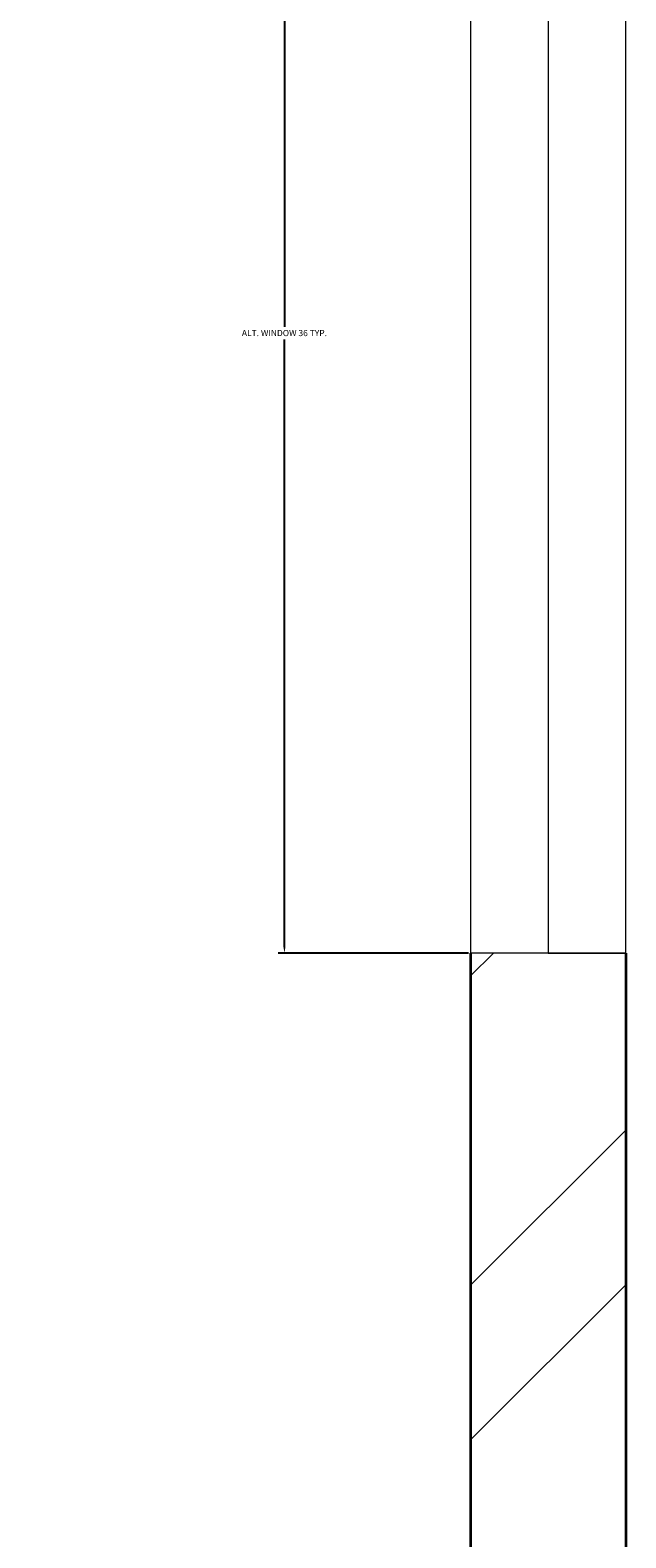
# Model space of a CAD drawing. Units: inches. Extents: x 1885 to 2748, y 783 to 2421.
# Tile 112 of 117: x 2601 to 2618, y 2027 to 2071. Entities that reach past the tile are written whole.
import ezdxf

# ---------------------------------------------------------------- set-up
doc = ezdxf.new("R2010")
doc.units = ezdxf.units.IN
for name, color, linetype, lineweight in [('A-ANNO-DIMS', 2, 'Continuous', 18), ('A-GLAZ', 181, 'Continuous', 18), ('A-WALL', 7, 'Continuous', 35)]:
    doc.layers.add(name, color=color, linetype=linetype, lineweight=lineweight)
doc.layers.add('A-WALL-PATT', color=85, linetype='Continuous', lineweight=13, true_color=0x58ba48)
doc.styles.get("Standard").update_dxf_attribs({"font": 'arial.ttf'})
doc.dimstyles.get("Standard").update_dxf_attribs({"dimtxt": 0.18, "dimasz": 0.18, "dimexe": 0.18, "dimexo": 0.0625, "dimgap": 0.09, "dimtad": 0, "dimtih": 1, "dimtoh": 1, "dimdec": 4, "dimzin": 0, "dimdsep": 46, "dimtxsty": 'Standard', "dimcen": 0.09, "dimadec": 0, "dimazin": 0, "dimtfac": 1, "dimtdec": 4, "dimtofl": 0, "dimtmove": 0, "dimatfit": 3, "dimfxl": 1, "dimtolj": 1, "dimtzin": 0, "dimarcsym": 0})

# ---------------------------------------------------------------- blocks, each defined once
blk = doc.blocks.new('WIN-36-ALT')
for p, q in [((0.004, 35.998), (4.504, 35.998)), ((0.004, 35.998), (0.004, -0.002)), ((4.504, 35.998), (2.254, 35.998)), ((2.254, 35.998), (2.254, -0.002)), ((4.504, -0.002), (4.504, 35.998)), ((4.504, -0.002), (0.004, -0.002)), ((2.254, -0.002), (4.504, -0.002))]:
    blk.add_line(p, q)
blk = doc.blocks.new('*D21')
at = {"layer": 'A-ANNO-DIMS', "color": 0, "lineweight": -2, "transparency": 16777216}
for p, q in [((2613.711, 2080.19), (2608.194, 2080.19)), ((2608.374, 2080.01), (2608.374, 2062.373)), ((2608.374, 2044.37), (2608.374, 2062.007)), ((2613.711, 2044.19), (2608.194, 2044.19))]:
    blk.add_line(p, q, dxfattribs=at)
at = {"layer": 'A-ANNO-DIMS', "color": 0, "transparency": 16777216}
for points in [[(2608.344, 2080.01), (2608.404, 2080.01), (2608.374, 2080.19)], [(2608.344, 2044.37), (2608.404, 2044.37), (2608.374, 2044.19)]]:
    blk.add_solid(points, dxfattribs=at)
at = {"layer": 'Defpoints', "color": 0, "transparency": 16777216}
for p in [(2608.374, 2080.19), (2613.774, 2080.19), (2613.774, 2044.19)]:
    blk.add_point(p, dxfattribs=at)
at = {"layer": 'A-ANNO-DIMS', "color": 0, "transparency": 16777216, "insert": (2608.374, 2062.19), "char_height": 0.18, "attachment_point": 5}
blk.add_mtext('\\A1;ALT. WINDOW 36 TYP.', dxfattribs=at)

msp = doc.modelspace()

# ---------------------------------------------------------------- hatches: boundary and pattern name
at = {"layer": 'A-WALL-PATT'}
h = msp.add_hatch(dxfattribs=at)
h.set_pattern_fill('ANSI32', color=256)
h.paths.add_polyline_path([(2007.772, 2318.006), (1980.774, 2318.006), (1980.774, 2281.215), (1985.274, 2281.215), (1985.274, 2313.506), (2007.772, 2313.506), (2007.772, 2315.756)])
h.paths.add_polyline_path([(2094.324, 2318.006), (2067.772, 2318.006), (2067.772, 2313.506), (2094.324, 2313.506), (2094.324, 2315.756)])
h.paths.add_polyline_path([(2131.367, 2315.756), (2131.367, 2318.006), (2131.189, 2318.006), (2112.609, 2318.006), (2112.609, 2313.506), (2117.274, 2313.506), (2117.274, 2255.201), (2121.774, 2255.201), (2121.774, 2313.506), (2131.367, 2313.506)])
h.paths.add_polyline_path([(2190.512, 2318.006), (2155.367, 2318.006), (2155.367, 2313.506), (2169.774, 2313.506), (2169.774, 2229.506), (2121.774, 2229.506), (2121.774, 2233.451), (2119.524, 2233.451), (2117.274, 2233.451), (2117.274, 2201.101), (2121.774, 2201.101), (2121.774, 2225.006), (2169.774, 2225.006), (2169.774, 2165.006), (2306.274, 2165.006), (2306.274, 2066.006), (2310.774, 2066.006), (2344.274, 2066.006), (2486.274, 2066.006), (2486.274, 1886.006), (2483.02, 1886.006), (2483.02, 1881.506), (2486.274, 1881.506), (2486.274, 1880.678), (2490.774, 1880.678), (2490.774, 2070.506), (2344.274, 2070.506), (2310.774, 2070.506), (2310.774, 2165.006), (2310.774, 2173.636), (2308.524, 2173.636), (2306.274, 2173.636), (2306.274, 2169.506), (2174.274, 2169.506), (2174.274, 2313.506), (2190.512, 2313.506), (2190.512, 2315.756)])
h.paths.add_polyline_path([(1985.274, 2221.215), (1980.774, 2221.215), (1980.774, 2165.006), (1992.774, 2165.006), (1992.774, 2141.927), (1997.274, 2141.927), (1997.274, 2165.006), (2117.274, 2165.006), (2117.274, 2163.126), (2121.774, 2163.126), (2121.774, 2172.734), (2119.524, 2172.734), (2117.274, 2172.734), (2117.274, 2169.506), (1985.274, 2169.506)])
h.paths.add_polyline_path([(1997.274, 2105.927), (1992.774, 2105.927), (1992.774, 2070.506), (2016.774, 2070.506), (2016.774, 2059.123), (2019.024, 2059.123), (2021.274, 2059.123), (2021.274, 2070.506), (2117.274, 2070.506), (2117.274, 2022.506), (2114.423, 2022.506), (2114.423, 2018.006), (2123.627, 2018.006), (2123.627, 2020.256), (2123.627, 2022.506), (2121.774, 2022.506), (2121.774, 2142.587), (2119.524, 2142.587), (2117.274, 2142.587), (2117.274, 2075.006), (1997.274, 2075.006)])
h.paths.add_polyline_path([(2092.029, 2020.256), (2092.029, 2022.506), (2021.274, 2022.506), (2021.274, 2035.123), (2016.774, 2035.123), (2016.774, 2018.006), (2016.774, 1978.784), (2021.274, 1978.784), (2021.274, 2018.006), (2092.029, 2018.006)])
h.paths.add_polyline_path([(2260.938, 2022.506), (2153.105, 2022.506), (2153.105, 2020.256), (2153.105, 2018.006), (2155.274, 2018.006), (2155.274, 1886.006), (2107.629, 1886.006), (2107.629, 1881.506), (2182.911, 1881.506), (2182.911, 1883.756), (2182.911, 1886.006), (2159.774, 1886.006), (2159.774, 2018.006), (2260.938, 2018.006), (2260.938, 2020.256)])
h.paths.add_polyline_path([(2047.629, 1883.756), (2047.629, 1886.006), (2021.274, 1886.006), (2021.274, 1918.784), (2019.024, 1918.784), (2016.774, 1918.784), (2016.774, 1881.506), (2047.629, 1881.506)])
h.paths.add_polyline_path([(2306.361, 1883.756), (2306.361, 1886.006), (2296.274, 1886.006), (2296.274, 1982.006), (2316.535, 1982.006), (2316.535, 1984.256), (2316.535, 1986.506), (2296.274, 1986.506), (2296.274, 2022.506), (2289.276, 2022.506), (2289.276, 2018.006), (2291.774, 2018.006), (2291.774, 1886.006), (2242.911, 1886.006), (2242.911, 1881.506), (2306.361, 1881.506)], flags=17)
h.paths.add_polyline_path([(1985.274, 1843.006), (2021.6, 1843.006), (2021.534, 1845.441), (2021.477, 1847.506), (1980.774, 1847.506), (1980.774, 1809.446), (1985.274, 1809.446)])
h.paths.add_polyline_path([(2131.482, 1845.256), (2131.482, 1847.506), (2081.534, 1847.506), (2081.534, 1843.006), (2117.274, 1843.006), (2117.274, 1784.147), (2119.524, 1784.147), (2121.774, 1784.147), (2121.774, 1843.006), (2131.482, 1843.006)])
h.paths.add_polyline_path([(2203.886, 1847.506), (2155.482, 1847.506), (2155.482, 1843.006), (2169.774, 1843.006), (2169.774, 1759.006), (2121.774, 1759.006), (2121.774, 1761.457), (2117.274, 1761.457), (2117.274, 1730.429), (2121.774, 1730.429), (2121.774, 1754.506), (2177.421, 1754.506), (2177.421, 1756.756), (2177.421, 1759.006), (2174.274, 1759.006), (2174.274, 1843.006), (2203.886, 1843.006)])
h.paths.add_polyline_path([(2335.554, 1845.256), (2335.554, 1847.506), (2239.886, 1847.506), (2239.886, 1843.006), (2306.274, 1843.006), (2306.274, 1759.006), (2199.486, 1759.006), (2199.486, 1754.506), (2310.774, 1754.506), (2310.774, 1843.006), (2335.554, 1843.006)])
h.paths.add_polyline_path([(2348.774, 2022.506), (2344.274, 2022.506), (2344.274, 1986.506), (2341.681, 1986.506), (2341.681, 1982.006), (2344.274, 1982.006), (2344.274, 1886.006), (2330.361, 1886.006), (2330.361, 1881.506), (2361.627, 1881.506), (2361.627, 1883.756), (2361.627, 1886.006), (2348.774, 1886.006)], flags=17)
h.paths.add_polyline_path([(2283.251, 2315.756), (2283.251, 2318.006), (2238.512, 2318.006), (2238.512, 2313.506), (2283.251, 2313.506)], flags=17)
h.paths.add_polyline_path([(2363.274, 2348.006), (2388.677, 2348.006), (2388.677, 2350.256), (2388.677, 2352.506), (2358.774, 2352.506), (2358.774, 2348.006), (2358.774, 2318.006), (2344.481, 2318.006), (2344.481, 2313.506), (2358.774, 2313.506), (2358.774, 2229.506), (2310.774, 2229.506), (2310.774, 2231.952), (2306.274, 2231.952), (2306.274, 2205.611), (2310.774, 2205.611), (2310.774, 2225.006), (2358.774, 2225.006), (2358.774, 2211.506), (2452.329, 2211.506), (2452.329, 2213.756), (2452.329, 2216.006), (2363.274, 2216.006), (2363.274, 2318.006)])
h.paths.add_polyline_path([(2310.774, 2313.506), (2320.481, 2313.506), (2320.481, 2315.756), (2320.481, 2318.006), (2302.728, 2318.006), (2302.728, 2313.506), (2306.274, 2313.506), (2306.274, 2251.076), (2310.774, 2251.076)], flags=17)
h.paths.add_polyline_path([(2490.774, 2352.506), (2486.274, 2352.506), (2448.677, 2352.506), (2448.677, 2348.006), (2486.274, 2348.006), (2486.274, 2318.006), (2486.274, 2216.006), (2481.78, 2216.006), (2481.78, 2211.506), (2486.274, 2211.506), (2486.274, 2165.006), (2493.289, 2165.006), (2493.289, 2167.256), (2493.289, 2169.506), (2490.774, 2169.506), (2490.774, 2313.506), (2494.429, 2313.506), (2494.429, 2318.006), (2490.774, 2318.006)])
h.paths.add_polyline_path([(2534.653, 2318.006), (2515.691, 2318.006), (2515.691, 2313.506), (2534.653, 2313.506), (2534.653, 2315.756)])
h.paths.add_polyline_path([(2618.274, 2318.006), (2594.653, 2318.006), (2594.653, 2313.506), (2613.774, 2313.506), (2613.774, 2281.706), (2618.274, 2281.706)])
h.paths.add_polyline_path([(2618.274, 2221.706), (2613.774, 2221.706), (2613.774, 2169.506), (2554.019, 2169.506), (2554.019, 2165.006), (2613.774, 2165.006), (2613.774, 2152.878), (2618.274, 2152.878)])
h.paths.add_polyline_path([(2618.274, 2128.878), (2616.024, 2128.878), (2613.774, 2128.878), (2613.774, 2117.006), (2529.774, 2117.006), (2529.774, 2165.006), (2532.848, 2165.006), (2532.848, 2169.506), (2522.867, 2169.506), (2522.867, 2165.006), (2525.274, 2165.006), (2525.274, 2117.006), (2525.274, 2112.506), (2525.274, 2108.576), (2529.774, 2108.576), (2529.774, 2112.506), (2613.774, 2112.506), (2613.774, 2080.19), (2618.274, 2080.19)])
h.paths.add_polyline_path([(2618.274, 2044.19), (2616.024, 2044.19), (2613.774, 2044.19), (2613.774, 2015.506), (2529.774, 2015.506), (2529.774, 2088.582), (2527.524, 2088.582), (2525.274, 2088.582), (2525.274, 2011.006), (2613.774, 2011.006), (2613.774, 1956.755), (2618.274, 1956.755)])
h.paths.add_polyline_path([(2618.274, 1881.506), (2618.274, 1896.755), (2613.774, 1896.755), (2613.774, 1881.506), (2613.774, 1847.506), (2592.715, 1847.506), (2592.715, 1843.006), (2613.774, 1843.006), (2613.774, 1765.006), (2613.774, 1760.506), (2609.621, 1760.506), (2609.621, 1756.006), (2613.774, 1756.006), (2613.774, 1660.006), (2608.544, 1660.006), (2608.544, 1655.506), (2613.774, 1655.506), (2613.774, 1508.158), (2618.274, 1508.158)])
h.paths.add_polyline_path([(2565.774, 1843.006), (2568.997, 1843.006), (2568.997, 1847.506), (2490.774, 1847.506), (2490.774, 1849.7), (2488.524, 1849.7), (2486.274, 1849.7), (2486.274, 1847.506), (2477.274, 1847.506), (2477.274, 1838.506), (2477.274, 1821.493), (2486.274, 1821.493), (2486.274, 1838.506), (2561.274, 1838.506), (2561.274, 1765.006), (2486.274, 1765.006), (2486.274, 1786.157), (2477.274, 1786.157), (2477.274, 1765.006), (2477.274, 1756.006), (2486.274, 1756.006), (2565.774, 1756.006), (2585.621, 1756.006), (2585.621, 1758.256), (2585.621, 1760.506), (2565.774, 1760.506), (2565.774, 1765.006)])
h.paths.add_polyline_path([(2486.274, 1651.006), (2561.274, 1651.006), (2561.274, 1567.006), (2486.274, 1567.006), (2486.274, 1591.321), (2477.274, 1591.321), (2477.274, 1567.006), (2477.274, 1558.006), (2477.274, 1555.439), (2481.774, 1555.439), (2481.774, 1558.006), (2568.653, 1558.006), (2568.653, 1560.256), (2568.653, 1562.506), (2565.774, 1562.506), (2565.774, 1655.506), (2584.544, 1655.506), (2584.544, 1657.756), (2584.544, 1660.006), (2565.774, 1660.006), (2486.274, 1660.006), (2477.274, 1660.006), (2477.274, 1651.006), (2477.274, 1632.989), (2486.274, 1632.989)])
h.paths.add_polyline_path([(2449.967, 1883.756), (2449.967, 1886.006), (2421.627, 1886.006), (2421.627, 1881.506), (2449.967, 1881.506)], flags=17)
h.paths.add_polyline_path([(2447.274, 1847.506), (2395.554, 1847.506), (2395.554, 1843.006), (2442.774, 1843.006), (2442.774, 1809.27), (2447.274, 1809.27)])
h.paths.add_polyline_path([(1985.274, 1749.446), (1980.774, 1749.446), (1980.774, 1694.504), (1985.274, 1694.504), (1985.274, 1694.506), (1986.897, 1694.506), (1986.897, 1697.78), (1986.897, 1699.006), (1985.274, 1699.006)])
h.paths.add_polyline_path([(2152.774, 1699.006), (2121.774, 1699.006), (2121.774, 1703.668), (2119.524, 1703.668), (2117.274, 1703.668), (2117.274, 1699.006), (2009.219, 1699.006), (2009.219, 1694.506), (2148.274, 1694.506), (2148.274, 1692.631), (2152.774, 1692.631)])
h.paths.add_polyline_path([(2016.274, 1694.506), (2011.774, 1694.506), (2011.774, 1558.006), (2040.806, 1558.006), (2040.806, 1560.256), (2040.806, 1562.506), (2016.274, 1562.506)])
h.paths.add_polyline_path([(2152.774, 1663.017), (2150.524, 1663.017), (2148.274, 1663.017), (2148.274, 1562.506), (2100.806, 1562.506), (2100.806, 1558.006), (2165.119, 1558.006), (2165.119, 1560.256), (2165.119, 1562.506), (2152.774, 1562.506), (2152.774, 1610.506), (2224.774, 1610.506), (2224.774, 1607.99), (2229.274, 1607.99), (2229.274, 1615.006), (2152.774, 1615.006)])
h.paths.add_polyline_path([(2238.613, 1560.256), (2238.613, 1562.506), (2229.274, 1562.506), (2229.274, 1588.756), (2227.024, 1588.763), (2224.774, 1588.771), (2224.774, 1562.506), (2189.119, 1562.506), (2189.119, 1558.006), (2238.613, 1558.006)])
h.paths.add_polyline_path([(2336.024, 1560.256), (2336.024, 1562.506), (2310.774, 1562.506), (2310.774, 1656.347), (2308.524, 1656.347), (2306.274, 1656.347), (2306.274, 1562.506), (2286.613, 1562.506), (2286.613, 1558.006), (2336.024, 1558.006)])
h.paths.add_polyline_path([(2447.274, 1690.968), (2445.024, 1690.968), (2442.774, 1690.968), (2442.774, 1687.006), (2306.274, 1687.006), (2306.274, 1680.75), (2310.774, 1680.75), (2310.774, 1682.506), (2442.774, 1682.506), (2442.774, 1562.506), (2396.024, 1562.506), (2396.024, 1558.006), (2447.274, 1558.006)])
h.paths.add_polyline_path([(2447.274, 1749.27), (2445.024, 1749.27), (2442.774, 1749.27), (2442.774, 1717.232), (2447.274, 1717.232)])
h.paths.add_polyline_path([(2044.674, 1521.756), (2044.674, 1524.006), (2007.274, 1524.006), (2007.274, 1503.49), (2009.524, 1503.49), (2011.774, 1503.49), (2011.774, 1519.506), (2044.674, 1519.506)])
h.paths.add_polyline_path([(2177.969, 1521.756), (2177.969, 1524.006), (2104.674, 1524.006), (2104.674, 1519.506), (2145.774, 1519.506), (2145.774, 1387.506), (2143.37, 1387.506), (2143.37, 1383.006), (2251.585, 1383.006), (2251.585, 1385.256), (2251.585, 1387.506), (2150.274, 1387.506), (2150.274, 1519.506), (2177.969, 1519.506)])
h.paths.add_polyline_path([(2298.704, 1524.006), (2237.969, 1524.006), (2237.969, 1519.506), (2282.274, 1519.506), (2282.274, 1387.506), (2279.683, 1387.506), (2279.683, 1383.006), (2286.774, 1383.006), (2286.774, 1419.006), (2312.451, 1419.006), (2312.451, 1421.256), (2312.451, 1423.506), (2286.774, 1423.506), (2286.774, 1519.506), (2298.704, 1519.506), (2298.704, 1521.722)], flags=17)
h.paths.add_polyline_path([(2361.897, 1521.756), (2361.897, 1524.006), (2322.704, 1524.006), (2322.704, 1519.506), (2334.774, 1519.506), (2334.774, 1423.506), (2331.93, 1423.506), (2331.93, 1419.006), (2334.774, 1419.006), (2334.774, 1387.506), (2334.774, 1383.228), (2339.274, 1383.228), (2339.274, 1387.506), (2339.274, 1519.506), (2361.897, 1519.506)], flags=17)
h.paths.add_polyline_path([(2447.274, 1521.756), (2447.274, 1524.006), (2421.897, 1524.006), (2421.897, 1519.506), (2447.274, 1519.506)], flags=17)
h.paths.add_polyline_path([(2481.774, 1529.6), (2479.524, 1529.6), (2477.274, 1529.6), (2477.274, 1524.006), (2474.489, 1524.006), (2474.489, 1519.506), (2477.274, 1519.506), (2477.274, 1334.506), (2296.774, 1334.506), (2296.774, 1240.506), (2160.274, 1240.506), (2160.274, 1180.506), (2112.274, 1180.506), (2112.274, 1207.692), (2110.024, 1207.692), (2107.774, 1207.692), (2107.774, 1171.609), (2112.274, 1171.609), (2112.274, 1176.006), (2160.274, 1176.006), (2160.274, 1092.006), (2144.221, 1092.006), (2144.221, 1087.506), (2189.497, 1087.506), (2189.497, 1089.756), (2189.497, 1092.006), (2164.774, 1092.006), (2164.774, 1236.006), (2296.774, 1236.006), (2296.774, 1231.912), (2301.274, 1231.912), (2301.274, 1330.006), (2481.774, 1330.006), (2481.774, 1387.506)])
h.paths.add_polyline_path([(2618.274, 1448.158), (2613.774, 1448.158), (2613.774, 1382.506), (2529.774, 1382.506), (2525.274, 1382.506), (2525.274, 1307.062), (2529.774, 1307.062), (2529.774, 1378.006), (2613.774, 1378.006), (2613.774, 1354.988), (2618.274, 1354.988)])
h.paths.add_polyline_path([(2618.274, 1318.988), (2613.774, 1318.988), (2613.774, 1281.006), (2529.774, 1281.006), (2529.774, 1283.786), (2527.524, 1283.786), (2525.274, 1283.786), (2525.274, 1228.506), (2516.794, 1228.506), (2516.794, 1224.006), (2533.484, 1224.006), (2533.484, 1226.256), (2533.484, 1228.506), (2529.774, 1228.506), (2529.774, 1276.506), (2613.774, 1276.506), (2613.774, 1266.02), (2618.274, 1266.02)])
h.paths.add_polyline_path([(2618.274, 1134.964), (2613.774, 1134.964), (2613.774, 1092.006), (2594.545, 1092.006), (2594.545, 1087.506), (2618.274, 1087.506)])
h.paths.add_polyline_path([(2534.545, 1092.006), (2509.765, 1092.006), (2509.765, 1087.506), (2534.545, 1087.506), (2534.545, 1089.756)])
h.paths.add_polyline_path([(2481.274, 1224.006), (2484.117, 1224.006), (2484.117, 1226.256), (2484.117, 1228.506), (2476.774, 1228.506), (2476.774, 1198.506), (2471.61, 1198.506), (2471.61, 1194.006), (2476.774, 1194.006), (2476.774, 1062.006), (2436.894, 1062.006), (2436.894, 1057.506), (2476.774, 1057.506), (2481.274, 1057.506), (2481.274, 1062.006), (2481.274, 1087.506), (2485.354, 1087.506), (2485.354, 1089.756), (2485.354, 1092.006), (2481.274, 1092.006), (2481.274, 1117.506)])
h.paths.add_polyline_path([(2439.898, 1198.506), (2349.274, 1198.506), (2349.274, 1194.006), (2349.274, 1180.506), (2301.274, 1180.506), (2301.274, 1201.896), (2299.024, 1201.896), (2296.774, 1201.896), (2296.774, 1172.335), (2299.024, 1172.335), (2301.274, 1172.335), (2301.274, 1176.006), (2349.274, 1176.006), (2349.274, 1092.006), (2334.452, 1092.006), (2334.452, 1087.506), (2349.274, 1087.506), (2349.274, 1057.506), (2353.774, 1057.506), (2376.894, 1057.506), (2376.894, 1059.756), (2376.894, 1062.006), (2353.774, 1062.006), (2353.774, 1087.506), (2353.774, 1180.506), (2353.774, 1194.006), (2439.898, 1194.006), (2439.898, 1196.256)])
h.paths.add_polyline_path([(2270.596, 1089.756), (2270.596, 1092.006), (2249.497, 1092.006), (2249.497, 1087.506), (2270.596, 1087.506)], flags=17)
h.paths.add_polyline_path([(2310.452, 1092.006), (2301.274, 1092.006), (2301.274, 1153.292), (2296.774, 1153.292), (2296.774, 1092.006), (2293.786, 1092.006), (2293.786, 1087.506), (2310.452, 1087.506), (2310.452, 1089.756)], flags=17)
h.paths.add_polyline_path([(2112.274, 1150.328), (2110.024, 1150.328), (2107.774, 1150.328), (2107.774, 1092.006), (2104.465, 1092.006), (2104.465, 1087.506), (2120.221, 1087.506), (2120.221, 1089.756), (2120.221, 1092.006), (2112.274, 1092.006)])
h.paths.add_polyline_path([(2082.172, 1092.006), (2058.144, 1092.006), (2058.144, 1087.506), (2082.172, 1087.506), (2082.172, 1089.756)])
h.paths.add_polyline_path([(1975.774, 1145.638), (1971.274, 1145.638), (1971.274, 1087.506), (1980.774, 1087.506), (1998.144, 1087.506), (1998.144, 1089.756), (1998.144, 1092.006), (1985.274, 1092.006), (1975.774, 1092.006)])
h.paths.add_polyline_path([(2112.274, 1244.385), (2110.024, 1244.385), (2107.774, 1244.385), (2107.774, 1240.506), (1992.274, 1240.506), (1992.274, 1271.008), (1987.774, 1271.008), (1987.774, 1240.506), (1980.774, 1240.506), (1975.774, 1240.506), (1971.274, 1240.506), (1971.274, 1205.638), (1975.774, 1205.638), (1975.774, 1236.006), (2107.774, 1236.006), (2107.774, 1233.444), (2112.274, 1233.444), (2112.274, 1236.006)])
h.paths.add_polyline_path([(2112.274, 1383.006), (2114.783, 1383.006), (2114.783, 1385.256), (2114.783, 1387.506), (2102.476, 1387.506), (2102.476, 1383.006), (2107.774, 1383.006), (2107.774, 1335.006), (2011.774, 1335.006), (2011.774, 1349.939), (2007.274, 1349.939), (2007.274, 1335.006), (1987.774, 1335.006), (1987.774, 1330.506), (1987.774, 1307.008), (1992.274, 1307.008), (1992.274, 1330.506), (2007.274, 1330.506), (2107.774, 1330.506), (2107.774, 1264.711), (2112.274, 1264.711)])
h.paths.add_polyline_path([(2077.857, 1387.506), (2011.774, 1387.506), (2011.774, 1390.036), (2009.524, 1390.036), (2007.274, 1390.036), (2007.274, 1373.939), (2011.774, 1373.939), (2011.774, 1383.006), (2077.857, 1383.006)])
h.paths.add_polyline_path([(2011.774, 1443.49), (2007.274, 1443.49), (2007.274, 1410.248), (2011.774, 1410.248)])

# ---------------------------------------------------------------- linework, layer by layer
at = {"layer": 'A-WALL'}
for p, q in [((2613.774, 2044.19), (2613.774, 2015.506)), ((2618.274, 2044.19), (2618.274, 1956.755))]:
    msp.add_line(p, q, dxfattribs=at)

# ---------------------------------------------------------------- block references
at = {"layer": 'A-GLAZ'}
msp.add_blockref('WIN-36-ALT', (2613.77, 2044.192), dxfattribs=at)

# ---------------------------------------------------------------- dimensions: what is measured, and where the dimension line sits
at = {"layer": 'A-ANNO-DIMS'}
dim = msp.add_linear_dim(base=(2608.374, 2080.19), p1=(2613.774, 2044.19), p2=(2613.774, 2080.19), angle=90, text='ALT. WINDOW <> TYP.', dimstyle='Standard', override={"dimdec": 0, "dimlfac": 1, "dimrnd": 0, "dimzin": 0, "dimdsep": 46, "dimlunit": 2}, dxfattribs=at)
dim.commit()
dim.dimension.update_dxf_attribs({"geometry": '*D21', "text_midpoint": (2608.374, 2062.19)})

doc.saveas('drawing.dxf')
